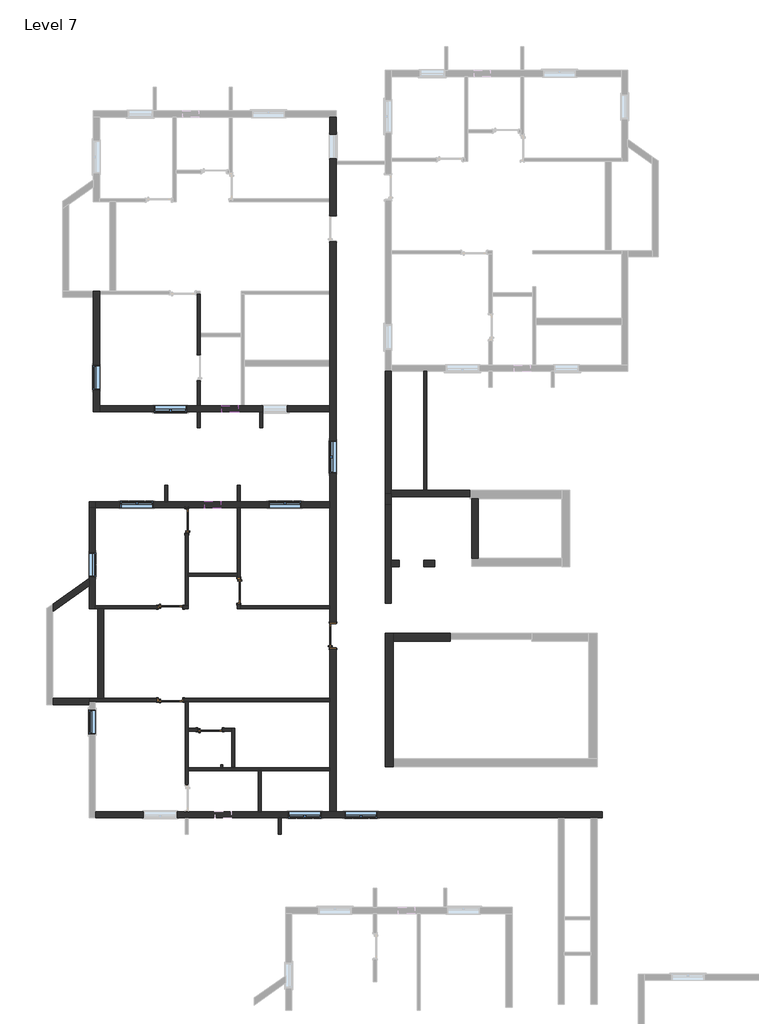
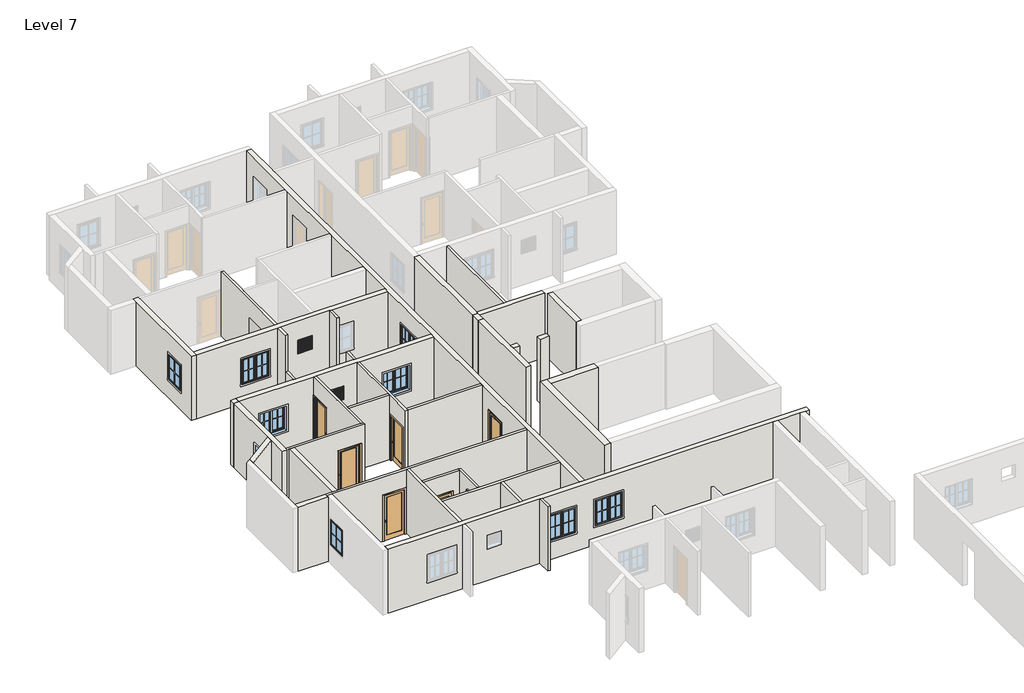
# One storey, part 4 of 7: 38 walls, 11 windows, 6 doors.
# Revit data of these elements (continued)
# Element 46 (IfcWindow, "Window-Awning-Single : 36\" x 48\"") (continued)
#   Mark = "153"
#   Window Inset = 0' - 0"
#   Interior Wall Closure = 0' - 2 1/4"
#   Frame Extension = 0' - 0 1/4"
#   Exterior Wall Closure = 0' - 1 1/4"
#   Interior Trim Visibility = yes
#   Exterior Trim Visibility = yes
#   Phase Created = New Construction
#   Materials on its faces: "Wood - Stained", "Glass", "Clad - White"
# Element 47 (IfcWindow, "Window-Awning-Single : 36\" x 48\"")
#   Mark = "165"
#   Window Inset = 0' - 0"
#   Interior Wall Closure = 0' - 2 1/4"
#   Frame Extension = 0' - 0 1/4"
#   Exterior Wall Closure = 0' - 1 1/4"
#   Interior Trim Visibility = yes
#   Exterior Trim Visibility = yes
#   Phase Created = New Construction
#   Materials on its faces: "Wood - Stained", "Glass", "Clad - White"
# Element 48 (IfcWindow, "Window-Casement-Double : 4' x 4'")
#   Mark = "168"
#   Window Inset = 0' - 0"
#   Interior Wall Closure = 0' - 2 1/4"
#   Frame Extension = 0' - 0 1/4"
#   Exterior Wall Closure = 0' - 1 1/4"
#   Interior Trim Visibility = yes
#   Exterior Trim Visibility = yes
#   Phase Created = New Construction
#   Materials on its faces: "Wood - Stained", "Glass", "Clad - White"
# Element 49 (IfcWindow, "Window-Casement-Double : 4' x 4'")
#   Mark = "193"
#   Window Inset = 0' - 0"
#   Interior Wall Closure = 0' - 2 1/4"
#   Frame Extension = 0' - 0 1/4"
#   Exterior Wall Closure = 0' - 1 1/4"
#   Interior Trim Visibility = yes
#   Exterior Trim Visibility = yes
#   Phase Created = New Construction
#   Materials on its faces: "Wood - Stained", "Glass", "Clad - White"
# Element 50 (IfcWindow, "Window-Casement-Double : 4' x 4'")
#   Mark = "194"
#   Window Inset = 0' - 0"
#   Interior Wall Closure = 0' - 2 1/4"
#   Frame Extension = 0' - 0 1/4"
#   Exterior Wall Closure = 0' - 1 1/4"
#   Interior Trim Visibility = yes
#   Exterior Trim Visibility = yes
#   Phase Created = New Construction
#   Materials on its faces: "Wood - Stained", "Glass", "Clad - White"
# Element 51 (IfcWindow, "Window-Casement-Double : 4' x 4'")
#   Mark = "196"
#   Window Inset = 0' - 0"
#   Interior Wall Closure = 0' - 2 1/4"
#   Frame Extension = 0' - 0 1/4"
#   Exterior Wall Closure = 0' - 1 1/4"
#   Interior Trim Visibility = yes
#   Exterior Trim Visibility = yes
#   Phase Created = New Construction
#   Materials on its faces: "Wood - Stained", "Glass", "Clad - White"
# Element 52 (IfcWindow, "Window-Casement-Double : 4' x 4'")
#   Mark = "197"
#   Window Inset = 0' - 0"
#   Interior Wall Closure = 0' - 2 1/4"
#   Frame Extension = 0' - 0 1/4"
#   Exterior Wall Closure = 0' - 1 1/4"
#   Interior Trim Visibility = yes
#   Exterior Trim Visibility = yes
#   Phase Created = New Construction
#   Materials on its faces: "Wood - Stained", "Glass", "Clad - White"
# Element 53 (IfcWindow, "Window-Casement-Double : 4' x 4'")
#   Mark = "198"
#   Window Inset = 0' - 0"
#   Interior Wall Closure = 0' - 2 1/4"
#   Frame Extension = 0' - 0 1/4"
#   Exterior Wall Closure = 0' - 1 1/4"
#   Interior Trim Visibility = yes
#   Exterior Trim Visibility = yes
#   Phase Created = New Construction
#   Materials on its faces: "Wood - Stained", "Glass", "Clad - White"
# Element 54 (IfcWindow, "Window-Louvers : 24\" x 24\"")
#   Mark = "134"
#   Blade Width = 1' - 10 1/2"
#   Phase Created = New Construction
#   Materials on its faces: "Birch"
# Element 55 (IfcWindow, "Window-Louvers : 24\" x 24\"")
#   Mark = "137"
#   Blade Width = 1' - 10 1/2"
#   Phase Created = New Construction
#   Materials on its faces: "Birch"
# Materials
#   "Cherry": class "Wood", colour RGB 226 177 128, transparency 0, Description = "Prunus Serotina", Cost = 0
#   "Aluminum": class "Metal", colour RGB 247 247 247, transparency 0, Description = "Aluminum 6061", Cost = 0
#   "Wood - Stained": class "Wood", colour RGB 224 178 126, transparency 0, Cost = 0
#   "Glass": class "Glass", colour RGB 0 128 192, transparency 0.75, Description = "Soda Lime Glass", Cost = 0
#   "Clad - White": class "Wood", colour RGB 242 242 238, transparency 0, Cost = 0
#   "Birch": class "Wood", colour RGB 224 178 126, transparency 0, Description = "Betula Alleghaniensis", Cost = 0
#   "Default Wall": colour RGB 128 128 128, transparency 0, Cost = 0
